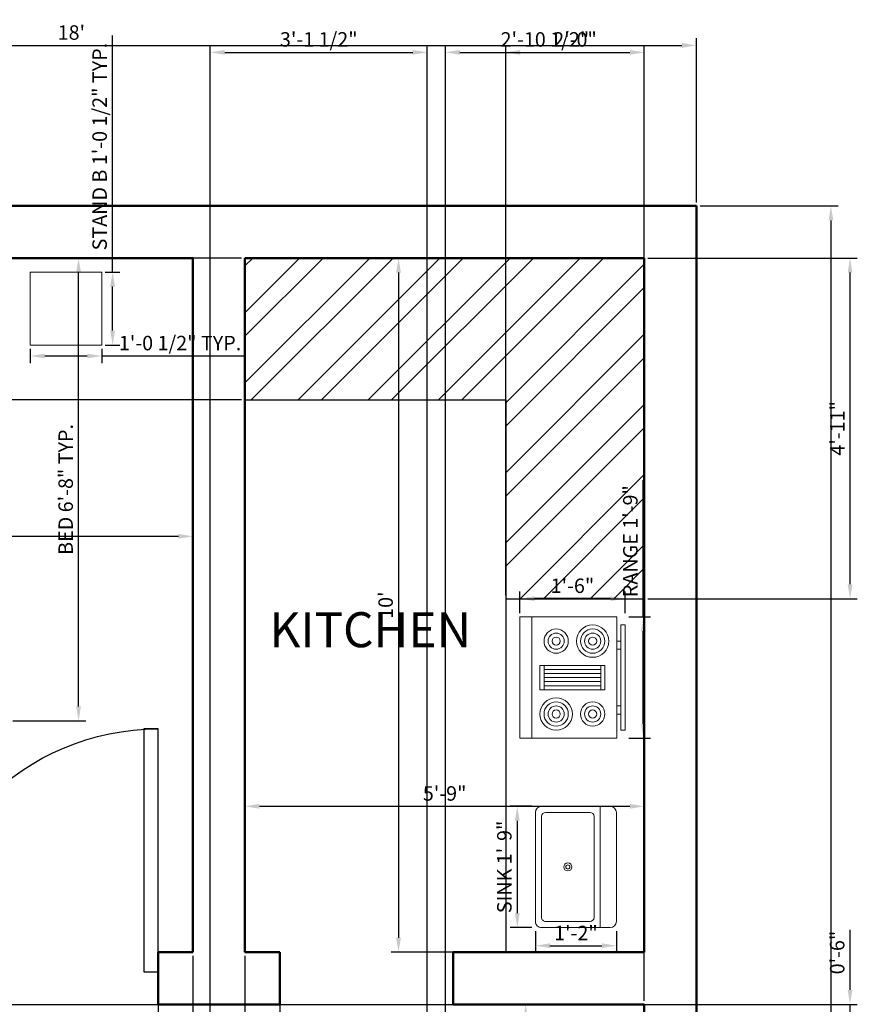
# Model space of a CAD drawing. Units: inches. Extents: x 1071 to 1348, y 2363 to 2916.
# Tile 4 of 4: x 1202 to 1347, y 2746 to 2916. Entities that reach past the tile are written whole.
import ezdxf

# ---------------------------------------------------------------- set-up
doc = ezdxf.new("R2010")
doc.units = ezdxf.units.IN
for name, color, linetype, lineweight in [('A-ANNO-DIMS', 2, 'Continuous', 18), ('A-AREA-IDEN', 7, 'Continuous', 25), ('A-DOOR', 4, 'Continuous', 25), ('A-EQPM', 8, 'Continuous', 20), ('A-FLOR-CASE', 9, 'Continuous', 25), ('A-FLOR-CASE-PATT', 252, 'Continuous', 13), ('A-FLOR-FIXT', 9, 'Continuous', 20), ('A-FURN', 8, 'Continuous', 18), ('A-WALL', 7, 'Continuous', 50)]:
    doc.layers.add(name, color=color, linetype=linetype, lineweight=lineweight)
doc.styles.get("Standard").update_dxf_attribs({"font": 'arial.ttf'})
doc.dimstyles.new('ISO-25', dxfattribs={"dimtxt": 2.5, "dimasz": 2.5, "dimexe": 1.25, "dimexo": 0.625, "dimtad": 1, "dimdec": 0, "dimlunit": 3, "dimtxsty": 'Standard', "dimcen": 2.5, "dimadec": 0, "dimazin": 0, "dimtfac": 1, "dimtdec": 0, "dimtmove": 0, "dimatfit": 3, "dimfxl": 1, "dimarcsym": 0})

# ---------------------------------------------------------------- blocks, each defined once
blk = doc.blocks.new('*U2')
for p, q in [((0, 0), (0, -100)), ((750, 0), (750, -100))]:
    blk.add_line(p, q)
blk.add_lwpolyline([(0, 0), (0, 750), (43.75, 750), (43.75, 0)], close=True)
blk.add_arc((0, 0), 750, 0, 90)
blk = doc.blocks.new('Range-Oven - 30 in top')
for p, q in [((0, -3), (30, -3)), ((12, -6), (18, -6)), ((13, -20), (13, -6)), ((14, -6), (14, -20)), ((15, -20), (15, -6)), ((16, -6), (16, -20)), ((17, -20), (17, -6)), ((18, -20), (12, -20)), ((6, -24), (6, -25)), ((8, -25), (8, -24)), ((22, -25), (22, -24)), ((24, -24), (24, -25))]:
    blk.add_line(p, q)
for points in [[(0, -24), (0, 0), (30, 0), (30, -24)], [(12, -21), (12, -5), (18, -5), (18, -21)], [(2, -26), (2, -25), (28, -25), (28, -26)]]:
    blk.add_lwpolyline(points, close=True)
for centre, radius in [((6, -9), 4), ((6, -9), 3), ((6, -9), 2), ((24, -9), 3), ((24, -9), 2), ((6, -9), 1), ((24, -9), 1), ((24, -18), 4), ((6, -18), 3), ((6, -18), 2), ((6, -18), 1), ((24, -18), 3), ((24, -18), 2), ((24, -18), 1)]:
    blk.add_circle(centre, radius)
blk = doc.blocks.new('Sink-single - 30 in top')
blk.add_line((-15, -3.999996), (15, -3.999996))
for points in [[(-13.5, 0), (13.5, 0)], [(-15, -18.499996), (-15, -1.5)], [(15, -1.5), (15, -18.499996)], [(-13.5, -17.499996), (-13.5, -6.499996)], [(-12.5, -5.499996), (12.5, -5.499996)], [(13.5, -6.499996), (13.5, -17.499996)], [(12.5, -18.499996), (-12.5, -18.499996)], [(13.5, -19.999996), (-13.5, -19.999996)]]:
    blk.add_lwpolyline(points)
for radius in [1, 0.5]:
    blk.add_circle((0, -11.999996), radius)
for centre, radius, start, end in [((-13.5, -1.5), 1.5, 90, 180), ((13.5, -1.5), 1.5, 0, 90), ((-12.5, -6.499996), 1, 90, 180), ((12.5, -6.499996), 1, 0, 90), ((-13.5, -18.499996), 1.5, 180, 270), ((-12.5, -17.499996), 1, 180, 270), ((12.5, -17.499996), 1, 270, 0), ((13.5, -18.499996), 1.5, 270, 0)]:
    blk.add_arc(centre, radius, start, end)
blk = doc.blocks.new('*D9')
at = {"layer": 'A-ANNO-DIMS', "color": 0, "lineweight": -2, "transparency": 16777216}
for p, q in [((1103.28, 2884.88), (1103.28, 2913.26)), ((1319.28, 2884.88), (1319.28, 2913.26)), ((1105.78, 2912.01), (1316.78, 2912.01))]:
    blk.add_line(p, q, dxfattribs=at)
at = {"layer": 'A-ANNO-DIMS', "color": 0, "transparency": 16777216}
for points in [[(1105.78, 2912.43), (1105.78, 2911.6), (1103.28, 2912.01)], [(1316.78, 2912.43), (1316.78, 2911.6), (1319.28, 2912.01)]]:
    blk.add_solid(points, dxfattribs=at)
at = {"layer": 'Defpoints', "color": 0, "transparency": 16777216}
for p in [(1319.28, 2912.01), (1103.28, 2884.25), (1319.28, 2884.25)]:
    blk.add_point(p, dxfattribs=at)
at = {"layer": 'A-ANNO-DIMS', "color": 0, "transparency": 16777216, "insert": (1211.28, 2913.91), "char_height": 2.5, "attachment_point": 5}
blk.add_mtext("18'", dxfattribs=at)
blk = doc.blocks.new('*D13')
at = {"layer": 'A-ANNO-DIMS', "color": 0, "lineweight": -2, "transparency": 16777216}
for p, q in [((1293.16, 2746.25), (1288.53, 2746.25)), ((1289.78, 2743.75), (1289.78, 2637.75)), ((1290.91, 2635.25), (1288.53, 2635.25))]:
    blk.add_line(p, q, dxfattribs=at)
at = {"layer": 'A-ANNO-DIMS', "color": 0, "transparency": 16777216}
for points in [[(1289.36, 2743.75), (1290.19, 2743.75), (1289.78, 2746.25)], [(1289.36, 2637.75), (1290.19, 2637.75), (1289.78, 2635.25)]]:
    blk.add_solid(points, dxfattribs=at)
at = {"layer": 'Defpoints', "color": 0, "transparency": 16777216}
for p in [(1293.78, 2746.25), (1289.78, 2635.25), (1291.53, 2635.25)]:
    blk.add_point(p, dxfattribs=at)
at = {"layer": 'A-ANNO-DIMS', "color": 0, "transparency": 16777216, "insert": (1287.87, 2690.75), "char_height": 2.5, "attachment_point": 5, "rotation": 90}
blk.add_mtext('9\'-3"', dxfattribs=at)
blk = doc.blocks.new('*D21')
at = {"layer": 'A-ANNO-DIMS', "color": 0, "lineweight": -2, "transparency": 16777216}
for p, q in [((1319.91, 2884.25), (1343.77, 2884.25)), ((1342.52, 2881.75), (1342.52, 2393.75)), ((1319.91, 2391.25), (1343.77, 2391.25))]:
    blk.add_line(p, q, dxfattribs=at)
at = {"layer": 'A-ANNO-DIMS', "color": 0, "transparency": 16777216}
for points in [[(1342.11, 2881.75), (1342.94, 2881.75), (1342.52, 2884.25)], [(1342.11, 2393.75), (1342.94, 2393.75), (1342.52, 2391.25)]]:
    blk.add_solid(points, dxfattribs=at)
at = {"layer": 'Defpoints', "color": 0, "transparency": 16777216}
for p in [(1319.28, 2884.25), (1319.28, 2391.25), (1342.52, 2391.25)]:
    blk.add_point(p, dxfattribs=at)
at = {"layer": 'A-ANNO-DIMS', "color": 0, "transparency": 16777216, "insert": (1340.64, 2637.75), "char_height": 2.5, "attachment_point": 5, "rotation": 90}
blk.add_mtext('41\'-1"', dxfattribs=at)
blk = doc.blocks.new('*D22')
at = {"layer": 'A-ANNO-DIMS', "color": 0, "lineweight": -2, "transparency": 16777216}
for p, q in [((1241.28, 2755.88), (1241.28, 2781.73)), ((1310.28, 2755.88), (1310.28, 2781.73)), ((1243.78, 2780.48), (1307.78, 2780.48))]:
    blk.add_line(p, q, dxfattribs=at)
at = {"layer": 'A-ANNO-DIMS', "color": 0, "transparency": 16777216}
for points in [[(1243.78, 2780.9), (1243.78, 2780.06), (1241.28, 2780.48)], [(1307.78, 2780.9), (1307.78, 2780.06), (1310.28, 2780.48)]]:
    blk.add_solid(points, dxfattribs=at)
at = {"layer": 'Defpoints', "color": 0, "transparency": 16777216}
for p in [(1310.28, 2780.48), (1241.28, 2755.25), (1310.28, 2755.25)]:
    blk.add_point(p, dxfattribs=at)
at = {"layer": 'A-ANNO-DIMS', "color": 0, "transparency": 16777216, "insert": (1275.78, 2782.38), "char_height": 2.5, "attachment_point": 5}
blk.add_mtext('5\'-9"', dxfattribs=at)
blk = doc.blocks.new('*D23')
at = {"layer": 'A-ANNO-DIMS', "color": 0, "lineweight": -2, "transparency": 16777216}
for p, q in [((1309.66, 2875.25), (1266.56, 2875.25)), ((1267.81, 2872.75), (1267.81, 2757.75)), ((1309.66, 2755.25), (1266.56, 2755.25))]:
    blk.add_line(p, q, dxfattribs=at)
at = {"layer": 'A-ANNO-DIMS', "color": 0, "transparency": 16777216}
for points in [[(1267.4, 2872.75), (1268.23, 2872.75), (1267.81, 2875.25)], [(1267.4, 2757.75), (1268.23, 2757.75), (1267.81, 2755.25)]]:
    blk.add_solid(points, dxfattribs=at)
at = {"layer": 'Defpoints', "color": 0, "transparency": 16777216}
for p in [(1310.28, 2875.25), (1267.81, 2755.25), (1310.28, 2755.25)]:
    blk.add_point(p, dxfattribs=at)
at = {"layer": 'A-ANNO-DIMS', "color": 0, "transparency": 16777216, "insert": (1265.91, 2815.25), "char_height": 2.5, "attachment_point": 5, "rotation": 90}
blk.add_mtext("10'", dxfattribs=at)
blk = doc.blocks.new('*D24')
at = {"layer": 'A-ANNO-DIMS', "color": 0, "lineweight": -2, "transparency": 16777216}
for p, q in [((1112.28, 2874.63), (1112.28, 2825.9)), ((1232.28, 2874.63), (1232.28, 2825.9)), ((1114.78, 2827.15), (1229.78, 2827.15))]:
    blk.add_line(p, q, dxfattribs=at)
at = {"layer": 'A-ANNO-DIMS', "color": 0, "transparency": 16777216}
for points in [[(1114.78, 2827.57), (1114.78, 2826.74), (1112.28, 2827.15)], [(1229.78, 2827.57), (1229.78, 2826.74), (1232.28, 2827.15)]]:
    blk.add_solid(points, dxfattribs=at)
at = {"layer": 'Defpoints', "color": 0, "transparency": 16777216}
for p in [(1112.28, 2875.25), (1232.28, 2875.25), (1232.28, 2827.15)]:
    blk.add_point(p, dxfattribs=at)
at = {"layer": 'A-ANNO-DIMS', "color": 0, "transparency": 16777216, "insert": (1172.28, 2829.06), "char_height": 2.5, "attachment_point": 5}
blk.add_mtext("10'", dxfattribs=at)
blk = doc.blocks.new('NIGHTSTAND-B')
blk.add_lwpolyline([(0, 0), (12.33, 0), (12.33, 12.6), (0, 12.6)], close=True)
blk = doc.blocks.new('*D29')
at = {"layer": 'A-ANNO-DIMS', "color": 0, "lineweight": -2, "transparency": 16777216}
for p, q in [((1201.15, 2875.25), (1213.78, 2875.25)), ((1212.53, 2797.75), (1212.53, 2872.75)), ((1201.15, 2795.25), (1213.78, 2795.25))]:
    blk.add_line(p, q, dxfattribs=at)
at = {"layer": 'A-ANNO-DIMS', "color": 0, "transparency": 16777216}
for points in [[(1212.11, 2872.75), (1212.94, 2872.75), (1212.53, 2875.25)], [(1212.11, 2797.75), (1212.94, 2797.75), (1212.53, 2795.25)]]:
    blk.add_solid(points, dxfattribs=at)
at = {"layer": 'Defpoints', "color": 0, "transparency": 16777216}
for p in [(1200.53, 2875.25), (1212.53, 2875.25), (1200.53, 2795.25)]:
    blk.add_point(p, dxfattribs=at)
at = {"layer": 'A-ANNO-DIMS', "color": 0, "transparency": 16777216, "insert": (1210.62, 2835.25), "char_height": 2.5, "attachment_point": 5, "rotation": 90}
blk.add_mtext('BED 6\'-8" TYP.', dxfattribs=at)
blk = doc.blocks.new('*D33')
at = {"layer": 'A-ANNO-DIMS', "color": 0, "lineweight": -2, "transparency": 16777216}
for p, q in [((1218.41, 2872.81), (1218.41, 2913.71)), ((1217.14, 2872.81), (1219.66, 2872.81)), ((1218.41, 2862.71), (1218.41, 2870.31)), ((1217.14, 2860.21), (1219.66, 2860.21))]:
    blk.add_line(p, q, dxfattribs=at)
at = {"layer": 'A-ANNO-DIMS', "color": 0, "transparency": 16777216}
for points in [[(1217.99, 2870.31), (1218.83, 2870.31), (1218.41, 2872.81)], [(1217.99, 2862.71), (1218.83, 2862.71), (1218.41, 2860.21)]]:
    blk.add_solid(points, dxfattribs=at)
at = {"layer": 'Defpoints', "color": 0, "transparency": 16777216}
for p in [(1216.52, 2872.81), (1218.41, 2872.81), (1216.52, 2860.21)]:
    blk.add_point(p, dxfattribs=at)
at = {"layer": 'A-ANNO-DIMS', "color": 0, "transparency": 16777216, "insert": (1216.49, 2894.51), "char_height": 2.5, "attachment_point": 5, "rotation": 90}
blk.add_mtext('STAND B 1\'-0 1/2" TYP.', dxfattribs=at)
blk = doc.blocks.new('*D34')
at = {"layer": 'A-ANNO-DIMS', "color": 0, "lineweight": -2, "transparency": 16777216}
for p, q in [((1204.19, 2859.58), (1204.19, 2857.07)), ((1216.52, 2859.58), (1216.52, 2857.07)), ((1206.69, 2858.32), (1214.02, 2858.32)), ((1216.52, 2858.32), (1241.1, 2858.32))]:
    blk.add_line(p, q, dxfattribs=at)
at = {"layer": 'A-ANNO-DIMS', "color": 0, "transparency": 16777216}
for points in [[(1206.69, 2858.73), (1206.69, 2857.9), (1204.19, 2858.32)], [(1214.02, 2858.73), (1214.02, 2857.9), (1216.52, 2858.32)]]:
    blk.add_solid(points, dxfattribs=at)
at = {"layer": 'Defpoints', "color": 0, "transparency": 16777216}
for p in [(1204.19, 2860.21), (1216.52, 2860.21), (1216.52, 2858.32)]:
    blk.add_point(p, dxfattribs=at)
at = {"layer": 'A-ANNO-DIMS', "color": 0, "transparency": 16777216, "insert": (1230.06, 2860.23), "char_height": 2.5, "attachment_point": 5}
blk.add_mtext('1\'-0 1/2" TYP.', dxfattribs=at)
blk = doc.blocks.new('*D41')
at = {"layer": 'A-ANNO-DIMS', "color": 0, "lineweight": -2, "transparency": 16777216}
for p, q in [((1310.11, 2813.23), (1310.11, 2836.88)), ((1307.58, 2813.23), (1311.36, 2813.23)), ((1310.11, 2794.73), (1310.11, 2810.73)), ((1307.58, 2792.23), (1311.36, 2792.23))]:
    blk.add_line(p, q, dxfattribs=at)
at = {"layer": 'A-ANNO-DIMS', "color": 0, "transparency": 16777216}
for points in [[(1309.69, 2810.73), (1310.52, 2810.73), (1310.11, 2813.23)], [(1309.69, 2794.73), (1310.52, 2794.73), (1310.11, 2792.23)]]:
    blk.add_solid(points, dxfattribs=at)
at = {"layer": 'Defpoints', "color": 0, "transparency": 16777216}
for p in [(1306.96, 2813.23), (1310.11, 2813.23), (1306.96, 2792.23)]:
    blk.add_point(p, dxfattribs=at)
at = {"layer": 'A-ANNO-DIMS', "color": 0, "transparency": 16777216, "insert": (1308.19, 2826.31), "char_height": 2.5, "attachment_point": 5, "rotation": 90}
blk.add_mtext('RANGE 1\'-9"', dxfattribs=at)
blk = doc.blocks.new('*D42')
at = {"layer": 'A-ANNO-DIMS', "color": 0, "lineweight": -2, "transparency": 16777216}
for p, q in [((1288.75, 2813.85), (1288.75, 2817.63)), ((1306.96, 2813.85), (1306.96, 2817.63)), ((1304.46, 2816.38), (1291.25, 2816.38))]:
    blk.add_line(p, q, dxfattribs=at)
at = {"layer": 'A-ANNO-DIMS', "color": 0, "transparency": 16777216}
for points in [[(1291.25, 2816.79), (1291.25, 2815.96), (1288.75, 2816.38)], [(1304.46, 2816.79), (1304.46, 2815.96), (1306.96, 2816.38)]]:
    blk.add_solid(points, dxfattribs=at)
at = {"layer": 'Defpoints', "color": 0, "transparency": 16777216}
for p in [(1288.75, 2816.38), (1288.75, 2813.23), (1306.96, 2813.23)]:
    blk.add_point(p, dxfattribs=at)
at = {"layer": 'A-ANNO-DIMS', "color": 0, "transparency": 16777216, "insert": (1297.86, 2818.28), "char_height": 2.5, "attachment_point": 5}
blk.add_mtext('1\'-6"', dxfattribs=at)
blk = doc.blocks.new('*D43')
at = {"layer": 'A-ANNO-DIMS', "color": 0, "lineweight": -2, "transparency": 16777216}
for p, q in [((1290.85, 2780.48), (1287.08, 2780.48)), ((1288.33, 2777.98), (1288.33, 2762.03)), ((1290.85, 2759.53), (1287.08, 2759.53))]:
    blk.add_line(p, q, dxfattribs=at)
at = {"layer": 'A-ANNO-DIMS', "color": 0, "transparency": 16777216}
for points in [[(1287.92, 2777.98), (1288.75, 2777.98), (1288.33, 2780.48)], [(1287.92, 2762.03), (1288.75, 2762.03), (1288.33, 2759.53)]]:
    blk.add_solid(points, dxfattribs=at)
at = {"layer": 'Defpoints', "color": 0, "transparency": 16777216}
for p in [(1291.48, 2780.48), (1288.33, 2759.53), (1291.48, 2759.53)]:
    blk.add_point(p, dxfattribs=at)
at = {"layer": 'A-ANNO-DIMS', "color": 0, "transparency": 16777216, "insert": (1286.42, 2770), "char_height": 2.5, "attachment_point": 5, "rotation": 90}
blk.add_mtext('SINK 1\'-9"', dxfattribs=at)
blk = doc.blocks.new('*D44')
at = {"layer": 'A-ANNO-DIMS', "color": 0, "lineweight": -2, "transparency": 16777216}
for p, q in [((1291.48, 2758.9), (1291.48, 2755.13)), ((1305.45, 2758.9), (1305.45, 2755.13)), ((1293.98, 2756.38), (1302.95, 2756.38))]:
    blk.add_line(p, q, dxfattribs=at)
at = {"layer": 'A-ANNO-DIMS', "color": 0, "transparency": 16777216}
for points in [[(1293.98, 2756.8), (1293.98, 2755.97), (1291.48, 2756.38)], [(1302.95, 2756.8), (1302.95, 2755.97), (1305.45, 2756.38)]]:
    blk.add_solid(points, dxfattribs=at)
at = {"layer": 'Defpoints', "color": 0, "transparency": 16777216}
for p in [(1291.48, 2759.53), (1305.45, 2759.53), (1305.45, 2756.38)]:
    blk.add_point(p, dxfattribs=at)
at = {"layer": 'A-ANNO-DIMS', "color": 0, "transparency": 16777216, "insert": (1298.46, 2758.26), "char_height": 2.5, "attachment_point": 5}
blk.add_mtext('1\'-2"', dxfattribs=at)
blk = doc.blocks.new('*D52')
at = {"layer": 'A-ANNO-DIMS', "color": 0, "lineweight": -2, "transparency": 16777216}
for p, q in [((1345.83, 2748.75), (1345.83, 2759.15)), ((1160.91, 2746.25), (1347.08, 2746.25)), ((1345.83, 2740.25), (1345.83, 2746.25)), ((1169.91, 2740.25), (1347.08, 2740.25)), ((1345.83, 2737.75), (1345.83, 2735.25))]:
    blk.add_line(p, q, dxfattribs=at)
at = {"layer": 'A-ANNO-DIMS', "color": 0, "transparency": 16777216}
for points in [[(1345.41, 2748.75), (1346.25, 2748.75), (1345.83, 2746.25)], [(1345.41, 2737.75), (1346.25, 2737.75), (1345.83, 2740.25)]]:
    blk.add_solid(points, dxfattribs=at)
at = {"layer": 'Defpoints', "color": 0, "transparency": 16777216}
for p in [(1160.28, 2746.25), (1345.83, 2746.25), (1169.28, 2740.25)]:
    blk.add_point(p, dxfattribs=at)
at = {"layer": 'A-ANNO-DIMS', "color": 0, "transparency": 16777216, "insert": (1343.93, 2755.2), "char_height": 2.5, "attachment_point": 5, "rotation": 90}
blk.add_mtext('0\'-6"', dxfattribs=at)
blk = doc.blocks.new('*D53')
at = {"layer": 'A-ANNO-DIMS', "color": 0, "lineweight": -2, "transparency": 16777216}
for p, q in [((1226.28, 2754.63), (1226.28, 2363.45)), ((1232.28, 2754.63), (1232.28, 2363.45)), ((1223.78, 2364.7), (1221.28, 2364.7)), ((1226.28, 2364.7), (1232.28, 2364.7)), ((1234.78, 2364.7), (1245.18, 2364.7))]:
    blk.add_line(p, q, dxfattribs=at)
at = {"layer": 'A-ANNO-DIMS', "color": 0, "transparency": 16777216}
for points in [[(1223.78, 2365.12), (1223.78, 2364.29), (1226.28, 2364.7)], [(1234.78, 2365.12), (1234.78, 2364.29), (1232.28, 2364.7)]]:
    blk.add_solid(points, dxfattribs=at)
at = {"layer": 'Defpoints', "color": 0, "transparency": 16777216}
for p in [(1226.28, 2755.25), (1232.28, 2755.25), (1232.28, 2364.7)]:
    blk.add_point(p, dxfattribs=at)
at = {"layer": 'A-ANNO-DIMS', "color": 0, "transparency": 16777216, "insert": (1241.23, 2366.61), "char_height": 2.5, "attachment_point": 5}
blk.add_mtext('0\'-6"', dxfattribs=at)
blk = doc.blocks.new('*D54')
at = {"layer": 'A-ANNO-DIMS', "color": 0, "lineweight": -2, "transparency": 16777216}
for p, q in [((1241.28, 2754.63), (1241.28, 2363.45)), ((1247.28, 2754.63), (1247.28, 2363.45)), ((1238.78, 2364.7), (1236.28, 2364.7)), ((1241.28, 2364.7), (1247.28, 2364.7)), ((1249.78, 2364.7), (1260.18, 2364.7))]:
    blk.add_line(p, q, dxfattribs=at)
at = {"layer": 'A-ANNO-DIMS', "color": 0, "transparency": 16777216}
for points in [[(1238.78, 2365.12), (1238.78, 2364.29), (1241.28, 2364.7)], [(1249.78, 2365.12), (1249.78, 2364.29), (1247.28, 2364.7)]]:
    blk.add_solid(points, dxfattribs=at)
at = {"layer": 'Defpoints', "color": 0, "transparency": 16777216}
for p in [(1241.28, 2755.25), (1247.28, 2755.25), (1247.28, 2364.7)]:
    blk.add_point(p, dxfattribs=at)
at = {"layer": 'A-ANNO-DIMS', "color": 0, "transparency": 16777216, "insert": (1256.23, 2366.61), "char_height": 2.5, "attachment_point": 5}
blk.add_mtext('0\'-6"', dxfattribs=at)
blk = doc.blocks.new('*D56')
at = {"layer": 'A-ANNO-DIMS', "color": 0, "lineweight": -2, "transparency": 16777216}
for p, q in [((1235.28, 2497.88), (1235.28, 2912.05)), ((1237.78, 2910.8), (1270.28, 2910.8)), ((1272.78, 2497.88), (1272.78, 2912.05))]:
    blk.add_line(p, q, dxfattribs=at)
at = {"layer": 'A-ANNO-DIMS', "color": 0, "transparency": 16777216}
for points in [[(1237.78, 2911.22), (1237.78, 2910.39), (1235.28, 2910.8)], [(1270.28, 2911.22), (1270.28, 2910.39), (1272.78, 2910.8)]]:
    blk.add_solid(points, dxfattribs=at)
at = {"layer": 'Defpoints', "color": 0, "transparency": 16777216}
for p in [(1272.78, 2910.8), (1235.28, 2497.25), (1272.78, 2497.25)]:
    blk.add_point(p, dxfattribs=at)
at = {"layer": 'A-ANNO-DIMS', "color": 0, "transparency": 16777216, "insert": (1254.03, 2912.72), "char_height": 2.5, "attachment_point": 5}
blk.add_mtext('3\'-1 1/2"', dxfattribs=at)
blk = doc.blocks.new('*D60')
at = {"layer": 'A-ANNO-DIMS', "color": 0, "lineweight": -2, "transparency": 16777216}
for p, q in [((1286.34, 2817), (1286.34, 2912.05)), ((1288.84, 2910.8), (1307.78, 2910.8)), ((1310.28, 2817), (1310.28, 2912.05))]:
    blk.add_line(p, q, dxfattribs=at)
at = {"layer": 'A-ANNO-DIMS', "color": 0, "transparency": 16777216}
for points in [[(1288.84, 2911.22), (1288.84, 2910.39), (1286.34, 2910.8)], [(1307.78, 2911.22), (1307.78, 2910.39), (1310.28, 2910.8)]]:
    blk.add_solid(points, dxfattribs=at)
at = {"layer": 'Defpoints', "color": 0, "transparency": 16777216}
for p in [(1310.28, 2910.8), (1286.34, 2816.37), (1310.28, 2816.37)]:
    blk.add_point(p, dxfattribs=at)
at = {"layer": 'A-ANNO-DIMS', "color": 0, "transparency": 16777216, "insert": (1298.31, 2912.71), "char_height": 2.5, "attachment_point": 5}
blk.add_mtext('2\'-0"', dxfattribs=at)
blk = doc.blocks.new('*D61')
at = {"layer": 'A-ANNO-DIMS', "color": 0, "lineweight": -2, "transparency": 16777216}
for p, q in [((1310.91, 2875.25), (1347.08, 2875.25)), ((1345.83, 2818.87), (1345.83, 2872.75)), ((1310.91, 2816.37), (1347.08, 2816.37))]:
    blk.add_line(p, q, dxfattribs=at)
at = {"layer": 'A-ANNO-DIMS', "color": 0, "transparency": 16777216}
for points in [[(1345.41, 2872.75), (1346.25, 2872.75), (1345.83, 2875.25)], [(1345.41, 2818.87), (1346.25, 2818.87), (1345.83, 2816.37)]]:
    blk.add_solid(points, dxfattribs=at)
at = {"layer": 'Defpoints', "color": 0, "transparency": 16777216}
for p in [(1310.28, 2875.25), (1345.83, 2875.25), (1310.28, 2816.37)]:
    blk.add_point(p, dxfattribs=at)
at = {"layer": 'A-ANNO-DIMS', "color": 0, "transparency": 16777216, "insert": (1343.95, 2845.81), "char_height": 2.5, "attachment_point": 5, "rotation": 90}
blk.add_mtext('4\'-11"', dxfattribs=at)
blk = doc.blocks.new('*D62')
at = {"layer": 'A-ANNO-DIMS', "color": 0, "lineweight": -2, "transparency": 16777216}
for p, q in [((1240.66, 2875.25), (1075.48, 2875.25)), ((1076.73, 2853.23), (1076.73, 2872.75)), ((1240.66, 2850.73), (1075.48, 2850.73))]:
    blk.add_line(p, q, dxfattribs=at)
at = {"layer": 'A-ANNO-DIMS', "color": 0, "transparency": 16777216}
for points in [[(1076.31, 2872.75), (1077.15, 2872.75), (1076.73, 2875.25)], [(1076.31, 2853.23), (1077.15, 2853.23), (1076.73, 2850.73)]]:
    blk.add_solid(points, dxfattribs=at)
at = {"layer": 'Defpoints', "color": 0, "transparency": 16777216}
for p in [(1076.73, 2875.25), (1241.28, 2875.25), (1241.28, 2850.73)]:
    blk.add_point(p, dxfattribs=at)
at = {"layer": 'A-ANNO-DIMS', "color": 0, "transparency": 16777216, "insert": (1074.81, 2862.99), "char_height": 2.5, "attachment_point": 5, "rotation": 90}
blk.add_mtext('2\'-0 1/2"', dxfattribs=at)
blk = doc.blocks.new('*D67')
at = {"layer": 'A-ANNO-DIMS', "color": 0, "lineweight": -2, "transparency": 16777216}
for p, q in [((1275.92, 2707.6), (1275.92, 2912.05)), ((1278.42, 2910.8), (1307.78, 2910.8)), ((1310.28, 2746.88), (1310.28, 2912.05))]:
    blk.add_line(p, q, dxfattribs=at)
at = {"layer": 'A-ANNO-DIMS', "color": 0, "transparency": 16777216}
for points in [[(1278.42, 2911.22), (1278.42, 2910.39), (1275.92, 2910.8)], [(1307.78, 2911.22), (1307.78, 2910.39), (1310.28, 2910.8)]]:
    blk.add_solid(points, dxfattribs=at)
at = {"layer": 'Defpoints', "color": 0, "transparency": 16777216}
for p in [(1310.28, 2910.8), (1310.28, 2746.25), (1275.92, 2706.97)]:
    blk.add_point(p, dxfattribs=at)
at = {"layer": 'A-ANNO-DIMS', "color": 0, "transparency": 16777216, "insert": (1293.1, 2912.72), "char_height": 2.5, "attachment_point": 5}
blk.add_mtext('2\'-10 1/2"', dxfattribs=at)

msp = doc.modelspace()

# ---------------------------------------------------------------- hatches: boundary and pattern name
at = {"layer": 'A-FLOR-CASE-PATT'}
h = msp.add_hatch(dxfattribs=at)
h.set_pattern_fill('ANSI32', color=256, scale=0.9)
h.paths.add_polyline_path([(1241.28, 2875.25), (1241.28, 2850.73), (1286.34, 2850.73), (1286.34, 2816.37), (1310.28, 2816.37), (1310.28, 2875.25)])
h.paths.add_polyline_path([(1243.95, 2806.31), (1284.21, 2806.31), (1284.21, 2815.7), (1243.95, 2815.7)], flags=9)

# ---------------------------------------------------------------- linework, layer by layer
at = {"layer": 'A-FLOR-CASE'}
for p, q in [((1241.28, 2850.73), (1286.34, 2850.73)), ((1286.34, 2850.73), (1286.34, 2755.25)), ((1286.34, 2816.37), (1310.28, 2816.37))]:
    msp.add_line(p, q, dxfattribs=at)
at = {"layer": 'A-WALL'}
for p, q in [((1103.28, 2884.25), (1319.28, 2884.25)), ((1319.28, 2884.25), (1319.28, 2391.25)), ((1112.28, 2875.25), (1232.28, 2875.25)), ((1232.28, 2875.25), (1232.28, 2755.25)), ((1241.28, 2875.25), (1241.28, 2755.25)), ((1241.28, 2875.25), (1310.28, 2875.25)), ((1310.28, 2875.25), (1310.28, 2755.25)), ((1226.28, 2755.25), (1226.28, 2746.25)), ((1226.28, 2755.25), (1232.28, 2755.25)), ((1241.28, 2755.25), (1247.28, 2755.25)), ((1247.28, 2755.25), (1247.28, 2746.25)), ((1277.28, 2755.25), (1277.28, 2746.25)), ((1277.28, 2755.25), (1310.28, 2755.25)), ((1226.28, 2746.25), (1247.28, 2746.25)), ((1277.28, 2746.25), (1310.28, 2746.25)), ((1310.28, 2746.25), (1310.28, 2635.25))]:
    msp.add_line(p, q, dxfattribs=at)

# ---------------------------------------------------------------- block references
at = {"layer": 'A-DOOR', "xscale": -0.0559999999999998, "yscale": 0.0559999999999998, "zscale": 0.0559999999999998}
msp.add_blockref('*U2', (1226.28, 2751.85), dxfattribs=at)
at = {"layer": 'A-EQPM', "xscale": 0.7000694306835537, "yscale": 0.7000694306835537, "zscale": 0.7000694306835537, "rotation": 90}
msp.add_blockref('Range-Oven - 30 in top', (1288.75, 2792.23), dxfattribs=at)
at = {"layer": 'A-FLOR-FIXT', "xscale": 0.6984764063607739, "yscale": 0.6984764063607739, "zscale": 0.6984764063607739, "rotation": 270}
msp.add_blockref('Sink-single - 30 in top', (1305.45, 2770), dxfattribs=at)
at = {"layer": 'A-FURN'}
msp.add_blockref('NIGHTSTAND-B', (1204.19, 2860.21), dxfattribs=at)

# ---------------------------------------------------------------- texts
at = {"layer": 'A-AREA-IDEN'}
msp.add_text('KITCHEN', height=6.055, dxfattribs=at).set_placement((1245.52, 2807.98))

# ---------------------------------------------------------------- dimensions: what is measured, and where the dimension line sits
at = {"layer": 'A-ANNO-DIMS'}
for base, p1, p2, override, picture, middle in [((1319.28, 2912.01), (1103.28, 2884.25), (1319.28, 2884.25), {"dimclrd": 0, "dimclre": 0, "dimclrt": 0}, '*D9', (1211.28, 2913.91)), ((1272.78, 2910.8), (1235.28, 2497.25), (1272.78, 2497.25), {"dimdec": 1, "dimlfac": 1, "dimrnd": 0, "dimzin": 1, "dimdsep": 46, "dimlunit": 4, "dimfrac": 2}, '*D56', (1254.03, 2912.72)), ((1310.28, 2910.8), (1275.92, 2706.97), (1310.28, 2746.25), {"dimdec": 1, "dimlfac": 1, "dimrnd": 0, "dimzin": 1, "dimdsep": 46, "dimlunit": 4, "dimfrac": 2}, '*D67', (1293.1, 2912.72)), ((1310.28, 2910.8), (1286.34, 2816.37), (1310.28, 2816.37), {"dimdec": 1, "dimlfac": 1, "dimrnd": 0, "dimzin": 1, "dimdsep": 46, "dimlunit": 4, "dimfrac": 2}, '*D60', (1298.31, 2912.71)), ((1232.28, 2827.15), (1112.28, 2875.25), (1232.28, 2875.25), {"dimclrd": 0, "dimclre": 0, "dimclrt": 0}, '*D24', (1172.28, 2829.06)), ((1310.28, 2780.48), (1241.28, 2755.25), (1310.28, 2755.25), {"dimclrd": 0, "dimclre": 0, "dimclrt": 0}, '*D22', (1275.78, 2782.38)), ((1305.45, 2756.38), (1291.48, 2759.53), (1305.45, 2759.53), {"dimdec": 1, "dimlfac": 1, "dimrnd": 0, "dimzin": 1, "dimdsep": 46, "dimlunit": 4, "dimfrac": 2}, '*D44', (1298.46, 2758.26)), ((1232.28, 2364.7), (1226.28, 2755.25), (1232.28, 2755.25), {"dimdec": 1, "dimlfac": 1, "dimrnd": 0, "dimzin": 1, "dimdsep": 46, "dimlunit": 4, "dimfrac": 2}, '*D53', (1241.23, 2366.61)), ((1247.28, 2364.7), (1241.28, 2755.25), (1247.28, 2755.25), {"dimdec": 1, "dimlfac": 1, "dimrnd": 0, "dimzin": 1, "dimdsep": 46, "dimlunit": 4, "dimfrac": 2}, '*D54', (1256.23, 2366.61))]:
    dim = msp.add_linear_dim(base=base, p1=p1, p2=p2, dimstyle='ISO-25', override=override, dxfattribs=at)
    dim.commit()
    dim.dimension.update_dxf_attribs({"geometry": picture, "text_midpoint": middle})
for base, p1, p2, angle, text, picture, middle in [((1218.41, 2872.81), (1216.52, 2860.21), (1216.52, 2872.81), 90, 'STAND B <> TYP.', '*D33', (1216.49, 2894.51)), ((1212.53, 2875.25), (1200.53, 2795.25), (1200.53, 2875.25), 90, 'BED <> TYP.', '*D29', (1210.62, 2835.25)), ((1310.11, 2813.23), (1306.96, 2792.23), (1306.96, 2813.23), 90, 'RANGE <>', '*D41', (1308.19, 2826.31)), ((1288.3341, 2759.5254), (1291.4772, 2780.4796), (1291.4772, 2759.5254), 270, 'SINK <>', '*D43', (1286.4165, 2770.0025))]:
    dim = msp.add_linear_dim(base=base, p1=p1, p2=p2, angle=angle, text=text, dimstyle='ISO-25', override={"dimdec": 1, "dimlfac": 1, "dimrnd": 0, "dimzin": 1, "dimdsep": 46, "dimlunit": 4, "dimfrac": 2}, dxfattribs=at)
    dim.commit()
    dim.dimension.update_dxf_attribs({"geometry": picture, "text_midpoint": middle})
for base, p1, p2, angle, override, picture, middle in [((1342.52, 2391.25), (1319.28, 2884.25), (1319.28, 2391.25), 90, {"dimclrd": 0, "dimclre": 0, "dimclrt": 0}, '*D21', (1340.64, 2637.75)), ((1076.73, 2875.25), (1241.28, 2850.73), (1241.28, 2875.25), 90, {"dimdec": 1, "dimlfac": 1, "dimrnd": 0, "dimzin": 1, "dimdsep": 46, "dimlunit": 4, "dimfrac": 2}, '*D62', (1074.81, 2862.99)), ((1267.81, 2755.25), (1310.28, 2875.25), (1310.28, 2755.25), 90, {"dimclrd": 0, "dimclre": 0, "dimclrt": 0}, '*D23', (1265.91, 2815.25)), ((1345.83, 2875.25), (1310.28, 2816.37), (1310.28, 2875.25), 90, {"dimdec": 1, "dimlfac": 1, "dimrnd": 0, "dimzin": 1, "dimdsep": 46, "dimlunit": 4, "dimfrac": 2}, '*D61', (1343.95, 2845.81)), ((1288.75, 2816.38), (1306.96, 2813.23), (1288.75, 2813.23), 180, {"dimdec": 1, "dimlfac": 1, "dimrnd": 0, "dimzin": 1, "dimdsep": 46, "dimlunit": 4, "dimfrac": 2}, '*D42', (1297.86, 2818.28)), ((1345.83, 2746.25), (1169.28, 2740.25), (1160.28, 2746.25), 90, {"dimdec": 1, "dimlfac": 1, "dimrnd": 0, "dimzin": 1, "dimdsep": 46, "dimlunit": 4, "dimfrac": 2}, '*D52', (1343.93, 2755.2)), ((1289.78, 2635.25), (1293.78, 2746.25), (1291.53, 2635.25), 90, {"dimclrd": 0, "dimclre": 0, "dimclrt": 0}, '*D13', (1287.87, 2690.75))]:
    dim = msp.add_linear_dim(base=base, p1=p1, p2=p2, angle=angle, dimstyle='ISO-25', override=override, dxfattribs=at)
    dim.commit()
    dim.dimension.update_dxf_attribs({"geometry": picture, "text_midpoint": middle})
dim = msp.add_linear_dim(base=(1216.52, 2858.32), p1=(1204.19, 2860.21), p2=(1216.52, 2860.21), text='<> TYP.', dimstyle='ISO-25', override={"dimdec": 1, "dimlfac": 1, "dimrnd": 0, "dimzin": 1, "dimdsep": 46, "dimlunit": 4, "dimfrac": 2}, dxfattribs=at)
dim.commit()
dim.dimension.update_dxf_attribs({"geometry": '*D34', "text_midpoint": (1230.06, 2860.23)})

doc.saveas('drawing.dxf')
